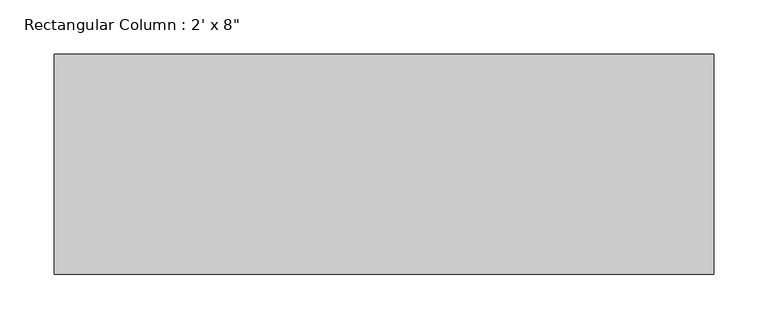
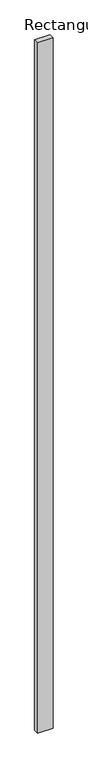
"""IFC4 building model written with IfcOpenShell, lengths in millimetres: column geometry."""

from ifc_helpers import new_model, si_unit, origin, origin_with_axes, place, context, project, spatial, polyline, outline, extrude, source, transform, mapped, element, save


def column_6d4d5e46(model_context):
    return source(origin(), model_context, "Body", "SweptSolid", [
        extrude(outline(polyline([(304.8, 101.6), (304.8, -101.6), (-304.8, -101.6), (-304.8, 101.6), (304.8, 101.6)])), origin_with_axes(), (0.0, 0.0, 1.0), 29108.4),
    ])


if __name__ == "__main__":
    model = new_model("IFC4")
    model_context = context("Model", 3, world=origin())
    ifc_project = project(units=[si_unit("LENGTHUNIT", "METRE", prefix="MILLI")], contexts=[model_context])
    site = spatial("IfcSite", under=ifc_project)
    building = spatial("IfcBuilding", under=site)
    placement = place(None, origin())
    column_shape = column_6d4d5e46(model_context)
    element("IfcColumn", 1, ObjectType="Rectangular Column : 2' x 8\"", at=placement, inside=building, context=model_context, shape_type="MappedRepresentation", body=[
        mapped(column_shape, transform((0.0, 0.0, 0.0), x_axis=(1.0, 0.0, 0.0), y_axis=(0.0, 1.0, 0.0), z_axis=(0.0, 0.0, 1.0))),
    ])
    save(model, "model.ifc")

# Revit data of these elements
# Type "Rectangular Column : 2' x 8\""
#   Assembly Code = "B1010200"
#   Depth = 0' - 8"
#   Offset Base = 0' - 0"
#   Offset Top = 0' - 0"
#   Width = 2' - 0"
#   Material = none
